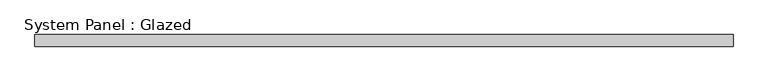
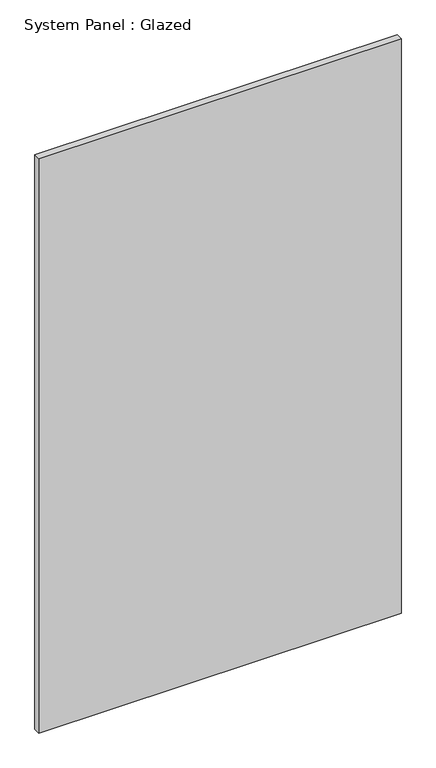
"""IFC4 building model written with IfcOpenShell, lengths in millimetres: plate geometry, System Panel : Glazed."""

from ifc_helpers import new_model, si_unit, origin, origin_with_axes, place, context, project, spatial, polyline, outline, extrude, source, transform, mapped, element, save


def system_panel_glazed_010dc334(model_context):
    return source(origin(), model_context, "Body", "SweptSolid", [
        extrude(outline(polyline([(734.390799, 19.05), (-734.390799, 19.05), (-734.390799, 44.45), (734.390799, 44.45), (734.390799, 19.05)])), origin_with_axes(), (0.0, 0.0, 1.0), 2460.728654),
    ])


if __name__ == "__main__":
    model = new_model("IFC4")
    model_context = context("Model", 3, world=origin())
    ifc_project = project(units=[si_unit("LENGTHUNIT", "METRE", prefix="MILLI")], contexts=[model_context])
    site = spatial("IfcSite", under=ifc_project)
    building = spatial("IfcBuilding", under=site)
    placement = place(None, origin())
    system_panel_glazed_shape = system_panel_glazed_010dc334(model_context)
    element("IfcPlate", 1, ObjectType="System Panel : Glazed", at=placement, inside=building, context=model_context, shape_type="MappedRepresentation", body=[
        mapped(system_panel_glazed_shape, transform((0.0, 0.0, 0.0), x_axis=(1.0, 0.0, 0.0), y_axis=(0.0, 1.0, 0.0), z_axis=(0.0, 0.0, 1.0))),
    ])
    save(model, "model.ifc")

# Revit data of these elements
# Type "System Panel : Glazed"
#   Construction Type Id = "GSP4R"
#   Analytic Construction = "1/8 in Pilkington single glazing"
#   Visual Light Transmittance = 0.9
#   Solar Heat Gain Coefficient = 0.86
#   Heat Transfer Coefficient (U) = 1.18115 BTU/(h·ft²·°F)
# Element 1 (IfcPlate, "System Panel : Glazed")
#   Materials on its faces: "Glass"
# Materials
#   "Glass": class "Glass", colour RGB 0 128 192, transparency 0.75, Description = "Soda Lime Glass", Cost = 0
